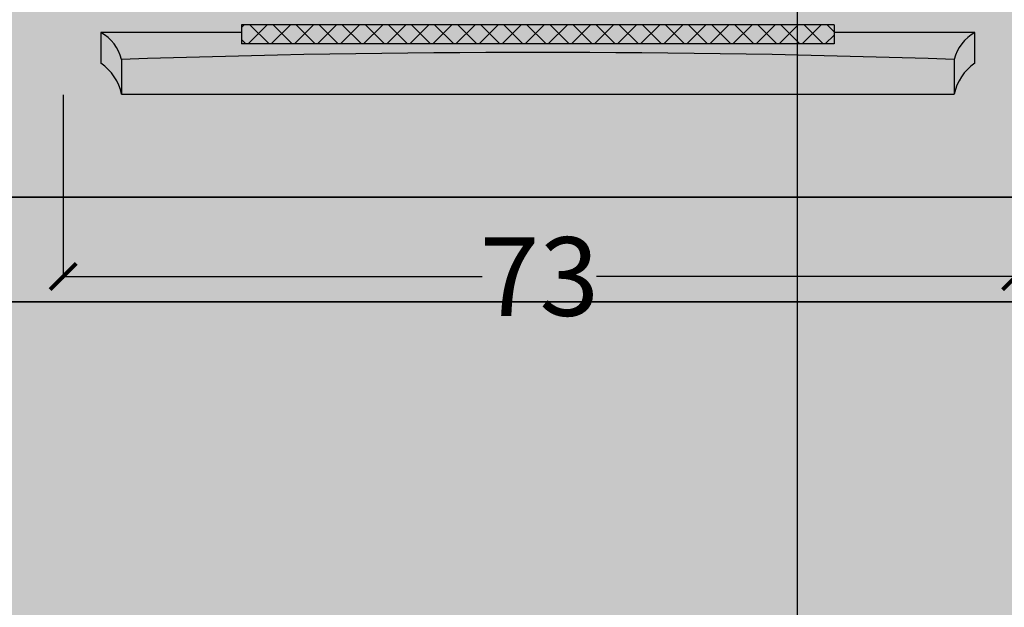
# Model space of a CAD drawing. Units: inches. Extents: x 1704 to 6393, y -157 to 1172.
# Tile 33 of 122: x 2488 to 2563, y 67 to 112. Entities that reach past the tile are written whole.
import ezdxf

# ---------------------------------------------------------------- set-up
doc = ezdxf.new("R2010")
doc.units = ezdxf.units.IN
doc.header["$MEASUREMENT"] = 0
for name, color, linetype, lineweight in [('A-ANNO-DIMS', 7, 'Continuous', 13), ('A-FURN', 8, 'Continuous', 18), ('A-WALL-PATT', 7, 'Continuous', 13), ('estofado', 7, 'Continuous', 25), ('WALLS', 7, 'Continuous', 35)]:
    doc.layers.add(name, color=color, linetype=linetype, lineweight=lineweight)
doc.layers.add('A-FLOR-PATT', color=7, linetype='Continuous', lineweight=13, true_color=0xf2f2f2)
doc.layers.add('L-HRDS-PATT', color=9, linetype='Continuous', lineweight=13, true_color=0xc5c1ba)
doc.styles.get("Standard").update_dxf_attribs({"font": 'arial.ttf'})
doc.dimstyles.get("Standard").update_dxf_attribs({"dimtxt": 6, "dimasz": 2, "dimexe": 0.18, "dimexo": 0.0625, "dimgap": 0.09, "dimtad": 0, "dimtih": 1, "dimtoh": 1, "dimdec": 1, "dimzin": 0, "dimdsep": 46, "dimlunit": 3, "dimtxsty": 'Standard', "dimblk": 'ARCHTICK', "dimcen": 0.09, "dimadec": 0, "dimazin": 0, "dimtfac": 1, "dimtdec": 1, "dimtofl": 0, "dimtmove": 0, "dimatfit": 3, "dimfxl": 1, "dimtolj": 1, "dimtzin": 0, "dimarcsym": 0})

# ---------------------------------------------------------------- blocks, each defined once
blk = doc.blocks.new('Cama Box Regencia LOLA')
at = {"layer": 'estofado', "ltscale": 0.2}
h = blk.add_hatch(color=256, dxfattribs=at)
h.dxf.hatch_style = 1
h.set_gradient(color1=(139, 102, 75), color2=(43, 31, 23), one_color=1, tint=0.13)
h.paths.add_polyline_path([(-0.8098, -0.0676), (-0.8098, 0, -0.197327), (-0.85, -0.06), (-0.85, -0.12, 0.208348)])
h = blk.add_hatch(color=256, dxfattribs=at)
h.dxf.hatch_style = 1
h.set_gradient(color1=(139, 102, 75), color2=(43, 31, 23), one_color=1, tint=0.13, name='CURVED')
h.paths.add_polyline_path([(0.8098, 0), (-0.8098, 0), (-0.8098, -0.0676, 0.016638), (0.8098, -0.0676)])
h = blk.add_hatch(color=256, dxfattribs=at)
h.dxf.hatch_style = 1
h.set_gradient(color1=(139, 102, 75), color2=(43, 31, 23), one_color=1, tint=0.13)
h.paths.add_polyline_path([(0.85, -0.06, -0.197327), (0.8098, 0), (0.8098, -0.0676, 0.208348), (0.85, -0.12)])
h = blk.add_hatch(color=256, dxfattribs=at)
h.dxf.hatch_style = 1
h.set_gradient(color1=(139, 102, 75), color2=(43, 31, 23), one_color=1, tint=0.13, name='INVCURVED')
h.paths.add_polyline_path([(0.8098, -0.0676, -0.016638), (-0.8098, -0.0676, -0.208348), (-0.85, -0.12), (-0.5763, -0.12), (-0.5763, -0.0977), (0.5763, -0.0977), (0.5763, -0.12), (0.85, -0.12, -0.208348)])
h = blk.add_hatch(color=256, dxfattribs=at)
h.dxf.hatch_style = 1
h.set_gradient(color1=(139, 102, 75), color2=(198, 169, 149), one_color=1, tint=0.68, name='CYLINDER')
h.paths.add_polyline_path([(0.5763, -0.0977), (-0.5763, -0.0977), (-0.5763, -0.1348), (0.5763, -0.1348)])
h = blk.add_hatch(dxfattribs=at)
h.set_pattern_fill('ANSI37,_O', color=256, scale=0.01)
h.set_pattern_definition([(45, (-24.743682, -44.176127), (-0.02245064, 0.02245064), []), (135, (-24.743682, -44.176127), (-0.02245064, -0.02245064), [])])
h.paths.add_polyline_path([(0.5763, -0.0977), (-0.5763, -0.0977), (-0.5763, -0.1348), (0.5763, -0.1348)])
for p, q in [((-0.8098, -0.0676), (-0.8098, 0)), ((0.8098, -0.0676), (0.8098, 0)), ((-0.5763, -0.0977), (0.5763, -0.0977)), ((-0.5763, -0.1348), (-0.5763, -0.0977)), ((0.5763, -0.1348), (0.5763, -0.0977)), ((-0.5763, -0.1348), (0.5763, -0.1348))]:
    blk.add_line(p, q, dxfattribs=at)
for points in [[(0.8098, 0), (-0.8098, 0)], [(-0.85, -0.06), (-0.85, -0.12), (-0.5763, -0.12)], [(0.5763, -0.12), (0.85, -0.12), (0.85, -0.06)]]:
    blk.add_lwpolyline(points, dxfattribs=at)
for centre, radius, start, end in [((-0.9029, 0.019), 0.0951, 303.8271, 348.4775), ((0.9029, 0.019), 0.0951, 191.5225, 236.1729), ((-0.89, -0.0476), 0.0827, 298.9176, 345.9939), ((0, 24.2598), 24.3409, 268.09356, 271.90644), ((0.89, -0.0476), 0.0827, 194.0061, 241.0824)]:
    blk.add_arc(centre, radius, start, end, dxfattribs=at)
blk = doc.blocks.new('_ArchTick')
at = {"color": 0, "linetype": 'ByBlock', "const_width": 0.15}
blk.add_lwpolyline([(-0.5, -0.5), (0.5, 0.5)], dxfattribs=at)
blk = doc.blocks.new('*D65')
at = {"layer": 'A-ANNO-DIMS', "color": 0, "lineweight": -2, "transparency": 16777216}
for p, q in [((2491.351, 106), (2491.351, 91.974)), ((2564.026, 106), (2564.026, 91.974)), ((2491.351, 92.154), (2523.326, 92.154)), ((2564.026, 92.154), (2532.051, 92.154))]:
    blk.add_line(p, q, dxfattribs=at)
at = {"layer": 'Defpoints', "color": 0, "lineweight": -3, "transparency": 16777216}
for p in [(2491.351, 106.063), (2564.026, 106.063), (2491.351, 92.154)]:
    blk.add_point(p, dxfattribs=at)
at = {"layer": 'A-ANNO-DIMS', "color": 0, "lineweight": -2, "transparency": 16777216, "xscale": 2, "yscale": 2, "zscale": 2, "rotation": 180}
blk.add_blockref('_ArchTick', (2491.351, 92.154), dxfattribs=at)
at = {"layer": 'A-ANNO-DIMS', "color": 0, "lineweight": -2, "transparency": 16777216, "xscale": 2, "yscale": 2, "zscale": 2}
blk.add_blockref('_ArchTick', (2564.026, 92.154), dxfattribs=at)
at = {"layer": 'A-ANNO-DIMS', "color": 0, "transparency": 16777216, "insert": (2527.689, 92.154), "char_height": 6, "attachment_point": 5}
blk.add_mtext('\\A1;73', dxfattribs=at)
blk = doc.blocks.new('*D93')
at = {"layer": 'A-ANNO-DIMS', "color": 0, "lineweight": -2, "transparency": 16777216}
for p, q in [((2605.286, 895.213), (1829.698, 895.213)), ((1829.878, 895.213), (1829.878, 495.866)), ((1829.878, 90.213), (1829.878, 489.56)), ((2605.286, 90.213), (1829.698, 90.213))]:
    blk.add_line(p, q, dxfattribs=at)
at = {"layer": 'Defpoints', "color": 0, "lineweight": -3, "transparency": 16777216}
for p in [(2605.349, 895.213), (1829.878, 90.213), (2605.349, 90.213)]:
    blk.add_point(p, dxfattribs=at)
at = {"layer": 'A-ANNO-DIMS', "color": 0, "lineweight": -2, "transparency": 16777216, "xscale": 2, "yscale": 2, "zscale": 2}
for p, rotation in [((1829.878, 895.213), 90), ((1829.878, 90.213), 270)]:
    blk.add_blockref('_ArchTick', p, dxfattribs=dict(at, rotation=rotation))
at = {"layer": 'A-ANNO-DIMS', "color": 0, "transparency": 16777216, "insert": (1829.878, 492.713), "char_height": 6, "attachment_point": 5}
blk.add_mtext('\\A1;805', dxfattribs=at)
blk = doc.blocks.new('*D105')
at = {"layer": 'A-ANNO-DIMS', "color": 0, "lineweight": -2, "transparency": 16777216}
for p, q in [((2451.738, 615.15), (2451.738, -64.967)), ((2547.349, 615.15), (2547.349, -64.967)), ((2451.738, -64.787), (2489.909, -64.787)), ((2547.349, -64.787), (2509.178, -64.787))]:
    blk.add_line(p, q, dxfattribs=at)
at = {"layer": 'Defpoints', "color": 0, "lineweight": -3, "transparency": 16777216}
for p in [(2451.738, 615.213), (2547.349, 615.213), (2547.349, -64.787)]:
    blk.add_point(p, dxfattribs=at)
at = {"layer": 'A-ANNO-DIMS', "color": 0, "lineweight": -2, "transparency": 16777216, "xscale": 2, "yscale": 2, "zscale": 2, "rotation": 180}
blk.add_blockref('_ArchTick', (2451.738, -64.787), dxfattribs=at)
at = {"layer": 'A-ANNO-DIMS', "color": 0, "lineweight": -2, "transparency": 16777216, "xscale": 2, "yscale": 2, "zscale": 2}
blk.add_blockref('_ArchTick', (2547.349, -64.787), dxfattribs=at)
at = {"layer": 'A-ANNO-DIMS', "color": 0, "transparency": 16777216, "insert": (2499.543, -64.787), "char_height": 6, "attachment_point": 5}
blk.add_mtext('\\A1;95.61', dxfattribs=at)

msp = doc.modelspace()

# ---------------------------------------------------------------- hatches: boundary and pattern name
at = {"layer": 'A-FLOR-PATT', "transparency": 33554528}
h = msp.add_hatch(color=256, dxfattribs=at)
h.dxf.hatch_style = 1
h.paths.add_polyline_path([(2325.349, 863.213), (2325.349, 887.213), (2263.349, 887.213), (2167.349, 887.213), (2081.349, 887.213), (2081.349, 719.213), (2277.349, 719.213), (2277.349, 711.213), (2277.349, 372.213), (2349.349, 372.213), (2381.349, 372.213), (2381.349, 364.213), (2353.349, 364.213), (2353.349, 270.213), (2381.349, 270.213), (2381.349, 266.213), (2357.349, 266.213), (2357.349, 98.213), (2381.349, 98.213), (2385.181, 98.213), (2386.482, 98.213), (2424.215, 98.213), (2425.516, 98.213), (2429.349, 98.213), (2597.349, 98.213), (2597.349, 146.213), (2597.349, 218.213), (2597.349, 266.213), (2423.349, 266.213), (2423.349, 270.213), (2473.349, 270.213), (2473.349, 294.213), (2477.349, 294.213), (2477.349, 270.213), (2547.349, 270.213), (2547.349, 364.213), (2477.349, 364.213), (2477.349, 318.213), (2473.349, 318.213), (2473.349, 364.213), (2423.349, 364.213), (2423.349, 372.213), (2469.349, 372.213), (2469.349, 459.213), (2469.349, 538.213), (2350.349, 538.213), (2350.349, 565.713), (2358.349, 565.713), (2358.349, 545.213), (2420.349, 545.213), (2420.349, 610.213), (2358.349, 610.213), (2358.349, 589.713), (2350.349, 589.713), (2350.349, 615.213), (2425.349, 615.213), (2425.349, 607.213), (2425.349, 546.213), (2469.349, 546.213), (2514.349, 546.213), (2514.349, 607.213), (2449.349, 607.213), (2449.349, 615.213), (2451.738, 615.213), (2451.738, 659.213), (2427.738, 659.213), (2427.738, 665.213), (2367.738, 665.213), (2367.738, 667.213), (2367.738, 711.213), (2325.349, 711.213), (2325.349, 719.213), (2325.349, 755.213), (2325.349, 763.213)])
h.paths.add_polyline_path([(2233.858, 822.533, -0.187247), (2233.858, 809.14), (2231.697, 808.804, 0.084893), (2233.131, 814.486), (2230.424, 814.486, -0.104258), (2228.553, 808.313), (2217.751, 807.156, -0.222222), (2217.751, 824.517), (2228.553, 823.359, -0.104258), (2230.424, 817.186), (2233.131, 817.186, 0.084893), (2231.697, 822.868)], flags=16)
h.paths.add_polyline_path([(2213.621, 833.197), (2213.621, 798.475), (2156.048, 798.475), (2156.048, 833.197)], flags=16)
h.paths.add_polyline_path([(2203.932, 848.099), (2205.089, 837.296, -0.222222), (2187.728, 837.296), (2188.885, 848.099, -0.104258), (2195.058, 849.969), (2195.058, 852.676, 0.084893), (2189.377, 851.242), (2189.712, 853.404, -0.187247), (2203.105, 853.404), (2203.44, 851.242, 0.084893), (2197.759, 852.676), (2197.759, 849.969, -0.104258)], flags=16)
h.paths.add_polyline_path([(2181.941, 837.296, -0.222222), (2164.58, 837.296), (2165.737, 848.099, -0.104258), (2171.91, 849.969), (2171.91, 852.676, 0.084893), (2166.229, 851.242), (2166.564, 853.404, -0.187247), (2179.957, 853.404), (2180.292, 851.242, 0.084893), (2174.611, 852.676), (2174.611, 849.969, -0.104258), (2180.784, 848.099)], flags=16)
h.paths.add_polyline_path([(2205.089, 794.376), (2203.932, 783.574, -0.104258), (2197.759, 781.703), (2197.759, 778.996, 0.084893), (2203.44, 780.43), (2203.105, 778.269, -0.187247), (2189.712, 778.269), (2189.377, 780.43, 0.084893), (2195.058, 778.996), (2195.058, 781.703, -0.104258), (2188.885, 783.574), (2187.728, 794.376, -0.222222)], flags=16)
h.paths.add_polyline_path([(2181.941, 794.376), (2180.784, 783.574, -0.104258), (2174.611, 781.703), (2174.611, 778.996, 0.084893), (2180.292, 780.43), (2179.957, 778.269, -0.187247), (2166.564, 778.269), (2166.229, 780.43, 0.084893), (2171.91, 778.996), (2171.91, 781.703, -0.104258), (2165.737, 783.574), (2164.58, 794.376, -0.222222)], flags=16)
h.paths.add_polyline_path([(2151.918, 807.156), (2141.116, 808.313, -0.104258), (2139.245, 814.486), (2136.539, 814.486, 0.084893), (2137.972, 808.804), (2135.811, 809.14, -0.187247), (2135.811, 822.533), (2137.972, 822.868, 0.084893), (2136.539, 817.186), (2139.245, 817.186, -0.104258), (2141.116, 823.359), (2151.918, 824.517, -0.222222)], flags=16)
h.paths.add_polyline_path([(2357.868, 363.41), (2358.814, 363.41, 0.75376)], flags=16)
h.paths.add_polyline_path([(2372.241, 363.117), (2372.248, 363.117), (2372.248, 363.343), (2371.302, 363.343), (2371.302, 363.139, -1.360391)], flags=16)
h.paths.add_polyline_path([(2371.309, 272.716), (2371.302, 272.716), (2371.302, 272.49), (2372.248, 272.49), (2372.248, 272.693, -1.360391)], flags=16)
h.paths.add_polyline_path([(2357.875, 272.716), (2357.868, 272.716), (2357.868, 272.49), (2358.814, 272.49), (2358.814, 272.693, -1.360391)], flags=16)
h.paths.add_polyline_path([(2353.769, 363.074), (2376.347, 363.074), (2376.347, 272.759), (2353.769, 272.759)], flags=16)
h.paths.add_polyline_path([(2354.772, 362.07), (2375.344, 362.07), (2375.344, 273.762), (2354.772, 273.762)], flags=0)
h.paths.add_polyline_path([(2357.868, 363.343), (2358.814, 363.343), (2358.814, 363.117), (2357.868, 363.117)], flags=16)
h.paths.add_polyline_path([(2359.288, 359.184), (2359.288, 360.063), (2370.828, 360.063), (2370.828, 359.184), (2374.332, 359.184), (2374.332, 358.464), (2372.835, 358.464), (2372.835, 357.541), (2374.332, 357.541), (2374.332, 356.82), (2372.835, 356.82), (2372.835, 355.898), (2374.332, 355.898), (2374.332, 355.177), (2372.835, 355.177), (2372.835, 354.254), (2374.332, 354.254), (2374.332, 353.534), (2372.835, 353.534), (2372.835, 352.611), (2374.332, 352.611), (2374.332, 351.89), (2372.835, 351.89), (2372.835, 350.968), (2374.332, 350.968), (2374.332, 350.247), (2372.835, 350.247), (2372.835, 349.324), (2374.332, 349.324), (2374.332, 348.604), (2372.835, 348.604), (2372.835, 347.681), (2374.332, 347.681), (2374.332, 346.96), (2372.835, 346.96), (2372.835, 346.038), (2374.332, 346.038), (2374.332, 345.317), (2372.835, 345.317), (2372.835, 344.395), (2374.332, 344.395), (2374.332, 343.674), (2372.835, 343.674), (2372.835, 342.751), (2374.332, 342.751), (2374.332, 342.03), (2372.835, 342.03), (2372.835, 341.108), (2374.332, 341.108), (2374.332, 340.387), (2372.835, 340.387), (2372.835, 339.465), (2374.332, 339.465), (2374.332, 338.744), (2372.835, 338.744), (2372.835, 337.821), (2374.332, 337.821), (2374.332, 337.1), (2372.835, 337.1), (2372.835, 336.178), (2374.332, 336.178), (2374.332, 335.457), (2372.835, 335.457), (2372.835, 334.535), (2374.332, 334.535), (2374.332, 333.814), (2372.835, 333.814), (2372.835, 332.891), (2374.332, 332.891), (2374.332, 332.171), (2372.835, 332.171), (2372.835, 331.248), (2374.332, 331.248), (2374.332, 330.527), (2372.835, 330.527), (2372.835, 329.605), (2374.332, 329.605), (2374.332, 328.884), (2372.835, 328.884), (2372.835, 327.961), (2374.332, 327.961), (2374.332, 327.241), (2372.835, 327.241), (2372.835, 326.318), (2374.332, 326.318), (2374.332, 325.597), (2372.835, 325.597), (2372.835, 324.675), (2374.332, 324.675), (2374.332, 323.954), (2372.835, 323.954), (2372.835, 323.031), (2374.332, 323.031), (2374.332, 322.311), (2372.835, 322.311), (2372.835, 321.388), (2374.332, 321.388), (2374.332, 320.667), (2372.835, 320.667), (2372.835, 319.745), (2374.332, 319.745), (2374.332, 319.024), (2372.835, 319.024), (2372.835, 318.102), (2374.332, 318.102), (2374.332, 317.381), (2372.835, 317.381), (2372.835, 316.458), (2374.332, 316.458), (2374.332, 315.737), (2372.835, 315.737), (2372.835, 314.815), (2374.332, 314.815), (2374.332, 314.094), (2372.835, 314.094), (2372.835, 313.172), (2374.332, 313.172), (2374.332, 312.451), (2372.835, 312.451), (2372.835, 311.528), (2374.332, 311.528), (2374.332, 310.807), (2372.835, 310.807), (2372.835, 309.885), (2374.332, 309.885), (2374.332, 309.164), (2372.835, 309.164), (2372.835, 308.242), (2374.332, 308.242), (2374.332, 307.521), (2372.835, 307.521), (2372.835, 306.598), (2374.332, 306.598), (2374.332, 305.878), (2372.835, 305.878), (2372.835, 304.955), (2374.332, 304.955), (2374.332, 304.234), (2372.835, 304.234), (2372.835, 303.312), (2374.332, 303.312), (2374.332, 302.591), (2372.835, 302.591), (2372.835, 301.668), (2374.332, 301.668), (2374.332, 300.948), (2372.835, 300.948), (2372.835, 300.025), (2374.332, 300.025), (2374.332, 299.304), (2372.835, 299.304), (2372.835, 298.382), (2374.332, 298.382), (2374.332, 297.661), (2372.835, 297.661), (2372.835, 296.738), (2374.332, 296.738), (2374.332, 296.018), (2372.835, 296.018), (2372.835, 295.095), (2374.332, 295.095), (2374.332, 294.374), (2372.835, 294.374), (2372.835, 293.452), (2374.332, 293.452), (2374.332, 292.731), (2372.835, 292.731), (2372.835, 291.809), (2374.332, 291.809), (2374.332, 291.088), (2372.835, 291.088), (2372.835, 290.165), (2374.332, 290.165), (2374.332, 289.444), (2372.835, 289.444), (2372.835, 288.522), (2374.332, 288.522), (2374.332, 287.801), (2372.835, 287.801), (2372.835, 286.879), (2374.332, 286.879), (2374.332, 286.158), (2372.835, 286.158), (2372.835, 285.235), (2374.332, 285.235), (2374.332, 284.514), (2372.835, 284.514), (2372.835, 283.592), (2374.332, 283.592), (2374.332, 282.871), (2372.835, 282.871), (2372.835, 281.949), (2374.332, 281.949), (2374.332, 281.228), (2372.835, 281.228), (2372.835, 280.305), (2374.332, 280.305), (2374.332, 279.585), (2372.835, 279.585), (2372.835, 278.662), (2374.332, 278.662), (2374.332, 277.941), (2372.835, 277.941), (2372.835, 277.019), (2374.332, 277.019), (2374.332, 276.298), (2370.828, 276.298), (2370.828, 275.769), (2359.288, 275.769), (2359.288, 276.298), (2355.784, 276.298), (2355.784, 277.019), (2357.281, 277.019), (2357.281, 277.941), (2355.784, 277.941), (2355.784, 278.662), (2357.281, 278.662), (2357.281, 279.585), (2355.784, 279.585), (2355.784, 280.305), (2357.281, 280.305), (2357.281, 281.228), (2355.784, 281.228), (2355.784, 281.949), (2357.281, 281.949), (2357.281, 282.871), (2355.784, 282.871), (2355.784, 283.592), (2357.281, 283.592), (2357.281, 284.514), (2355.784, 284.514), (2355.784, 285.235), (2357.281, 285.235), (2357.281, 286.158), (2355.784, 286.158), (2355.784, 286.879), (2357.281, 286.879), (2357.281, 287.801), (2355.784, 287.801), (2355.784, 288.522), (2357.281, 288.522), (2357.281, 289.444), (2355.784, 289.444), (2355.784, 290.165), (2357.281, 290.165), (2357.281, 291.088), (2355.784, 291.088), (2355.784, 291.809), (2357.281, 291.809), (2357.281, 292.731), (2355.784, 292.731), (2355.784, 293.452), (2357.281, 293.452), (2357.281, 294.374), (2355.784, 294.374), (2355.784, 295.095), (2357.281, 295.095), (2357.281, 296.018), (2355.784, 296.018), (2355.784, 296.738), (2357.281, 296.738), (2357.281, 297.661), (2355.784, 297.661), (2355.784, 298.382), (2357.281, 298.382), (2357.281, 299.304), (2355.784, 299.304), (2355.784, 300.025), (2357.281, 300.025), (2357.281, 300.948), (2355.784, 300.948), (2355.784, 301.668), (2357.281, 301.668), (2357.281, 302.591), (2355.784, 302.591), (2355.784, 303.312), (2357.281, 303.312), (2357.281, 304.234), (2355.784, 304.234), (2355.784, 304.955), (2357.281, 304.955), (2357.281, 305.878), (2355.784, 305.878), (2355.784, 306.598), (2357.281, 306.598), (2357.281, 307.521), (2355.784, 307.521), (2355.784, 308.242), (2357.281, 308.242), (2357.281, 309.164), (2355.784, 309.164), (2355.784, 309.885), (2357.281, 309.885), (2357.281, 310.807), (2355.784, 310.807), (2355.784, 311.528), (2357.281, 311.528), (2357.281, 312.451), (2355.784, 312.451), (2355.784, 313.172), (2357.281, 313.172), (2357.281, 314.094), (2355.784, 314.094), (2355.784, 314.815), (2357.281, 314.815), (2357.281, 315.737), (2355.784, 315.737), (2355.784, 316.458), (2357.281, 316.458), (2357.281, 317.381), (2355.784, 317.381), (2355.784, 318.102), (2357.281, 318.102), (2357.281, 319.024), (2355.784, 319.024), (2355.784, 319.745), (2357.281, 319.745), (2357.281, 320.667), (2355.784, 320.667), (2355.784, 321.388), (2357.281, 321.388), (2357.281, 322.311), (2355.784, 322.311), (2355.784, 323.031), (2357.281, 323.031), (2357.281, 323.954), (2355.784, 323.954), (2355.784, 324.675), (2357.281, 324.675), (2357.281, 325.597), (2355.784, 325.597), (2355.784, 326.318), (2357.281, 326.318), (2357.281, 327.241), (2355.784, 327.241), (2355.784, 327.961), (2357.281, 327.961), (2357.281, 328.884), (2355.784, 328.884), (2355.784, 329.605), (2357.281, 329.605), (2357.281, 330.527), (2355.784, 330.527), (2355.784, 331.248), (2357.281, 331.248), (2357.281, 332.171), (2355.784, 332.171), (2355.784, 332.891), (2357.281, 332.891), (2357.281, 333.814), (2355.784, 333.814), (2355.784, 334.535), (2357.281, 334.535), (2357.281, 335.457), (2355.784, 335.457), (2355.784, 336.178), (2357.281, 336.178), (2357.281, 337.1), (2355.784, 337.1), (2355.784, 337.821), (2357.281, 337.821), (2357.281, 338.744), (2355.784, 338.744), (2355.784, 339.465), (2357.281, 339.465), (2357.281, 340.387), (2355.784, 340.387), (2355.784, 341.108), (2357.281, 341.108), (2357.281, 342.03), (2355.784, 342.03), (2355.784, 342.751), (2357.281, 342.751), (2357.281, 343.674), (2355.784, 343.674), (2355.784, 344.395), (2357.281, 344.395), (2357.281, 345.317), (2355.784, 345.317), (2355.784, 346.038), (2357.281, 346.038), (2357.281, 346.96), (2355.784, 346.96), (2355.784, 347.681), (2357.281, 347.681), (2357.281, 348.604), (2355.784, 348.604), (2355.784, 349.324), (2357.281, 349.324), (2357.281, 350.247), (2355.784, 350.247), (2355.784, 350.968), (2357.281, 350.968), (2357.281, 351.89), (2355.784, 351.89), (2355.784, 352.611), (2357.281, 352.611), (2357.281, 353.534), (2355.784, 353.534), (2355.784, 354.254), (2357.281, 354.254), (2357.281, 355.177), (2355.784, 355.177), (2355.784, 355.898), (2357.281, 355.898), (2357.281, 356.82), (2355.784, 356.82), (2355.784, 357.541), (2357.281, 357.541), (2357.281, 358.464), (2355.784, 358.464), (2355.784, 359.184)], flags=0)
at = {"layer": 'A-WALL-PATT', "transparency": 33554643}
h = msp.add_hatch(color=256, dxfattribs=at)
h.dxf.hatch_style = 1
h.paths.add_polyline_path([(2167.349, 895.213), (2073.349, 895.213), (2073.349, 887.213), (2081.349, 887.213), (2167.349, 887.213)])
h.paths.add_polyline_path([(2465.349, 895.213), (2273.349, 895.213), (2273.349, 903.213), (2263.349, 903.213), (2263.349, 895.213), (2263.349, 887.213), (2325.349, 887.213), (2325.349, 863.213), (2333.349, 863.213), (2333.349, 887.213), (2465.349, 887.213)])
h.paths.add_polyline_path([(2533.349, 895.213), (2513.349, 895.213), (2513.349, 887.213), (2513.349, 861.213), (2517.349, 861.213), (2517.349, 887.213), (2533.349, 887.213)])
h.paths.add_polyline_path([(2605.349, 895.213), (2581.349, 895.213), (2581.349, 887.213), (2597.349, 887.213), (2597.349, 854.213), (2605.349, 854.213)])
h.paths.add_polyline_path([(2605.349, 752.213), (2629.349, 752.213), (2629.349, 716.213), (2605.349, 716.213), (2605.349, 712.213), (2719.349, 712.213), (2719.349, 716.213), (2631.349, 716.213), (2631.349, 754.213), (2605.349, 754.213), (2605.349, 794.213), (2597.349, 794.213), (2597.349, 787.213), (2517.349, 787.213), (2517.349, 813.213), (2513.349, 813.213), (2513.349, 783.213), (2517.349, 783.213), (2597.349, 783.213), (2597.349, 719.213), (2517.349, 719.213), (2517.349, 753.213), (2513.349, 753.213), (2513.349, 719.213), (2365.349, 719.213), (2365.349, 763.213), (2325.349, 763.213), (2325.349, 755.213), (2357.349, 755.213), (2357.349, 719.213), (2325.349, 719.213), (2325.349, 711.213), (2547.349, 711.213), (2547.349, 615.213), (2449.349, 615.213), (2449.349, 607.213), (2514.349, 607.213), (2514.349, 546.213), (2439.349, 546.213), (2425.349, 546.213), (2425.349, 607.213), (2425.349, 615.213), (2350.349, 615.213), (2350.349, 589.713), (2358.349, 589.713), (2358.349, 610.213), (2420.349, 610.213), (2420.349, 545.213), (2358.349, 545.213), (2358.349, 565.713), (2350.349, 565.713), (2350.349, 538.213), (2469.349, 538.213), (2469.349, 459.213), (2469.349, 372.213), (2423.349, 372.213), (2423.349, 364.213), (2473.349, 364.213), (2473.349, 318.213), (2477.349, 318.213), (2477.349, 364.213), (2547.349, 364.213), (2547.349, 352.213), (2549.349, 352.213), (2549.349, 364.213), (2597.349, 364.213), (2597.349, 328.213), (2549.349, 328.213), (2547.349, 328.213), (2547.349, 326.213), (2549.349, 326.213), (2597.349, 326.213), (2605.349, 326.213), (2605.349, 377.057), (2597.349, 377.057), (2597.349, 372.213), (2477.349, 372.213), (2477.349, 451.213), (2597.349, 451.213), (2605.349, 451.213), (2605.349, 459.213), (2597.349, 459.213), (2477.349, 459.213), (2477.349, 538.213), (2597.349, 538.213), (2597.349, 495.213), (2605.349, 495.213), (2605.349, 512.213), (2631.349, 512.213), (2631.349, 568.213), (2605.349, 568.213), (2605.349, 577.213), (2597.349, 577.213), (2597.349, 542.213), (2518.349, 542.213), (2518.349, 607.213), (2532.349, 607.213), (2605.349, 607.213), (2605.349, 615.213), (2597.349, 615.213), (2551.349, 615.213), (2551.349, 711.213), (2597.349, 711.213), (2597.349, 645.213), (2605.349, 645.213), (2605.349, 712.213), (2605.349, 716.213)])
h.paths.add_polyline_path([(2605.349, 566.213), (2629.349, 566.213), (2629.349, 514.213), (2605.349, 514.213)], flags=16)
h.paths.add_polyline_path([(2381.349, 372.213), (2349.349, 372.213), (2349.349, 202.213), (2337.349, 202.213), (2337.349, 194.213), (2349.349, 194.213), (2349.349, 90.213), (2349.349, 72.213), (2357.349, 72.213), (2357.349, 90.213), (2381.349, 90.213), (2381.349, 98.213), (2357.349, 98.213), (2357.349, 266.213), (2381.349, 266.213), (2381.349, 270.213), (2353.349, 270.213), (2353.349, 364.213), (2381.349, 364.213)])
h.paths.add_polyline_path([(2605.349, 302.213), (2597.349, 302.213), (2597.349, 270.213), (2477.349, 270.213), (2477.349, 294.213), (2473.349, 294.213), (2473.349, 270.213), (2423.349, 270.213), (2423.349, 266.213), (2597.349, 266.213), (2597.349, 218.213), (2605.349, 218.213)])
h.paths.add_polyline_path([(2605.349, 146.213), (2597.349, 146.213), (2597.349, 98.213), (2429.349, 98.213), (2429.349, 90.213), (2597.349, 90.213), (2597.349, 72.213), (2605.349, 72.213), (2605.349, 90.213)])
h.paths.add_polyline_path([(2225.349, 202.213), (2049.349, 202.213), (2049.349, 194.213), (2225.349, 194.213)])
h.paths.add_polyline_path([(2289.349, 202.213), (2277.349, 202.213), (2273.349, 202.213), (2269.516, 202.213), (2269.516, 194.213), (2273.349, 194.213), (2277.349, 194.213), (2289.349, 194.213)])
h.paths.add_polyline_path([(2273.349, 372.213), (2029.19, 372.213), (2029.19, 364.213), (2273.349, 364.213)])
h.paths.add_polyline_path([(2277.349, 545.213), (2213.349, 545.213), (2213.349, 573.213), (2205.349, 573.213), (2177.349, 573.213), (2177.349, 545.213), (2073.349, 545.213), (2073.349, 538.213), (2081.349, 538.213), (2277.349, 538.213)])
h.paths.add_polyline_path([(2181.349, 545.213), (2181.349, 569.213), (2205.349, 569.213), (2205.349, 545.213)], flags=16)
h.paths.add_polyline_path([(2277.349, 719.213), (2081.349, 719.213), (2073.349, 719.213), (2073.349, 711.213), (2154.575, 711.213), (2205.349, 711.213), (2205.349, 687.213), (2205.349, 629.213), (2213.349, 629.213), (2273.349, 629.213), (2273.349, 631.213), (2207.349, 631.213), (2207.349, 707.213), (2231.349, 707.213), (2231.349, 709.213), (2207.349, 709.213), (2207.349, 711.213), (2277.349, 711.213)])
at = {"layer": 'L-HRDS-PATT', "transparency": 33554539}
h = msp.add_hatch(color=256, dxfattribs=at)
h.dxf.hatch_style = 1
h.paths.add_polyline_path([(2651.217, 368.213), (2605.349, 368.213), (2605.349, 218.213), (2605.349, 212.464), (2605.349, 210.513), (2605.349, 153.913), (2605.349, 151.962), (2605.349, 146.213), (2605.349, 90.213), (2605.349, 72.213), (2601.349, 72.213), (2600.88, 50.634), (2719.349, 50.634), (2719.349, 72.213), (2711.349, 72.213), (2663.217, 72.213), (2651.217, 72.213)])
h.paths.add_polyline_path([(2711.349, 48.634), (2600.88, 48.634), (2576.88, 48.634), (2576.88, 17.658), (2711.349, 17.658)])
h.paths.add_polyline_path([(2601.349, 72.213), (2597.349, 72.213), (2597.349, 90.213), (2429.349, 90.213), (2425.516, 90.213), (2424.215, 90.213), (2386.482, 90.213), (2385.181, 90.213), (2381.349, 90.213), (2357.349, 90.213), (2357.349, 72.213), (2349.349, 72.213), (2349.349, 90.213), (2349.349, 134.213), (2277.349, 134.213), (2277.349, 50.634), (2566.88, 50.634), (2600.88, 50.634)])
h.paths.add_polyline_path([(2349.349, 146.213), (2277.349, 146.213), (2277.349, 134.213), (2349.349, 134.213)])
h.paths.add_polyline_path([(2349.349, 158.213), (2277.349, 158.213), (2277.349, 146.213), (2349.349, 146.213)])
h.paths.add_polyline_path([(2349.349, 170.213), (2277.349, 170.213), (2277.349, 158.213), (2349.349, 158.213)])
h.paths.add_polyline_path([(2349.349, 194.213), (2337.349, 194.213), (2337.349, 202.213), (2349.349, 202.213), (2349.349, 364.213), (2277.349, 364.213), (2277.349, 202.213), (2289.349, 202.213), (2289.349, 194.213), (2277.349, 194.213), (2277.349, 170.213), (2349.349, 170.213)])

# ---------------------------------------------------------------- linework, layer by layer
at = {"layer": 'WALLS'}
for p, q in [((2597.349, 98.213), (2429.349, 98.213)), ((2597.349, 90.213), (2429.349, 90.213))]:
    msp.add_line(p, q, dxfattribs=at)

# ---------------------------------------------------------------- block references
at = {"layer": 'A-FURN', "xscale": 39.22313671019584, "yscale": 39.22313671019584, "zscale": 39.22313671019584, "rotation": 180}
msp.add_blockref('Cama Box Regencia LOLA', (2527.569, 106.063), dxfattribs=at)

# ---------------------------------------------------------------- dimensions: what is measured, and where the dimension line sits
at = {"layer": 'A-ANNO-DIMS'}
for base, p1, p2, angle, picture, middle in [((1829.878, 90.213), (2605.349, 895.213), (2605.349, 90.213), 90, '*D93', (1829.878, 492.713)), ((2491.351, 92.154), (2564.026, 106.063), (2491.351, 106.063), 180, '*D65', (2527.689, 92.154))]:
    dim = msp.add_linear_dim(base=base, p1=p1, p2=p2, angle=angle, dimstyle='Standard', override={"dimdec": 0, "dimlfac": 1, "dimrnd": 0, "dimzin": 0, "dimdsep": 46, "dimlunit": 2}, dxfattribs=at)
    dim.commit()
    dim.dimension.update_dxf_attribs({"geometry": picture, "text_midpoint": middle})
dim = msp.add_linear_dim(base=(2547.349, -64.787), p1=(2451.738, 615.213), p2=(2547.349, 615.213), dimstyle='Standard', override={"dimdec": 2, "dimlfac": 1, "dimrnd": 0, "dimzin": 0, "dimdsep": 46, "dimlunit": 2}, dxfattribs=at)
dim.commit()
dim.dimension.update_dxf_attribs({"geometry": '*D105', "text_midpoint": (2499.543, -64.787)})

doc.saveas('drawing.dxf')
